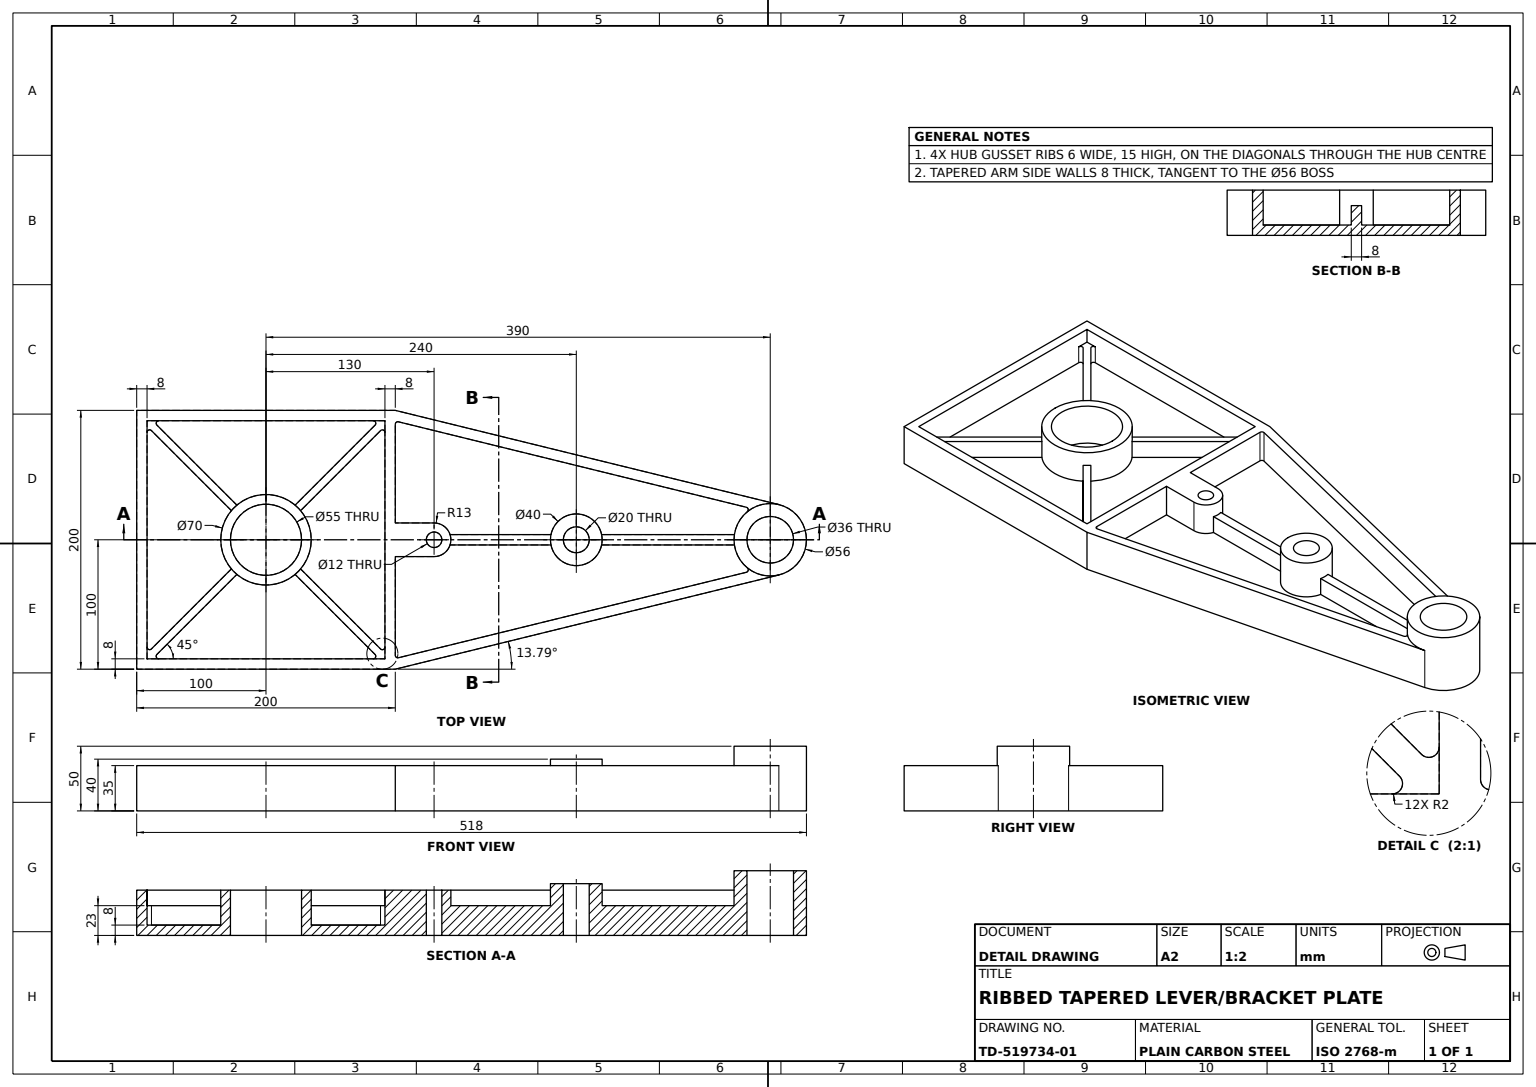
from build123d import *

# Parameters (mm, degrees)
BASE_PLATE_8MM_DEPTH      = 8
PERIMETER_WALL_SKETCH_W   = 200
PERIMETER_WALL_SKETCH_H   = 200
PERIMETER_WALL_SKETCH_W_2 = 184
PERIMETER_WALL_SKETCH_H_2 = 184
PERIMETER_WALL_DEPTH      = 27
CROSS_WALL_DEPTH          = 27
TIP_BOSS_SKETCH_R         = 28
ARM_TIP_BOSS_DEPTH        = 42
ARM_PAD_130X26_DEPTH      = 27
HUB_BOSS_SKETCH_R         = 35
HUB_BOSS_70_DEPTH         = 27
MID_BOSS_SKETCH_R         = 20
MID_ARM_BOSS_40_DEPTH     = 32
HUB_GUSSET_RIBS_4X_DEPTH  = 15
WALL_AND_RIB_FILLETS_R2_R = 2
ARM_RIBS_SKETCH_W         = 8
ARM_RIBS_SKETCH_H         = 265.57093639
ARM_GUSSET_RIBS_DEPTH     = 15
BOSS_BORES_SKETCH_R       = 27.5
BOSS_BORES_SKETCH_R_2     = 6
BOSS_BORES_SKETCH_R_3     = 10
BOSS_BORES_SKETCH_R_4     = 18
BOSS_BORES_DEPTH          = 433.693887177


with BuildPart() as part:
    # Base Plate Sketch → Base Plate 8mm (new body)
    with BuildSketch(Plane(origin=(0, 0, 0), x_dir=(1, 0, 0), z_dir=(0, 1, 0))):
        with BuildLine():
            Line((-100, -100), (100, -100))
            Line((100, -100), (100, 100))
            Line((100, 100), (27.193098987, 396.673482409))
            ThreePointArc((27.193098987, 396.673482409), (0, 418), (-27.193098987, 396.673482409))
            Line((-27.193098987, 396.673482409), (-100, 100))
            Line((-100, 100), (-100, -100))
        make_face()
    extrude(amount=BASE_PLATE_8MM_DEPTH)

    # Perimeter Wall Sketch → Perimeter Wall (add)
    with BuildSketch(Plane(origin=(0, 8, 0), x_dir=(1, 0, 0), z_dir=(0, 1, 0))):
        Rectangle(PERIMETER_WALL_SKETCH_W, PERIMETER_WALL_SKETCH_H)
        Rectangle(PERIMETER_WALL_SKETCH_W_2, PERIMETER_WALL_SKETCH_H_2, mode=Mode.SUBTRACT)
    extrude(amount=PERIMETER_WALL_DEPTH)

    # Cross Wall Sketch → Cross Wall (add)
    with BuildSketch(Plane(origin=(0, 8, 0), x_dir=(1, 0, 0), z_dir=(0, 1, 0))):
        with BuildLine():
            Line((-100, 100), (-27.193098987, 396.673482409))
            ThreePointArc((-27.193098987, 396.673482409), (0, 418), (27.193098987, 396.673482409))
            Line((27.193098987, 396.673482409), (100, 100))
            Line((100, 100), (100, 92))
            Line((100, 92), (-100, 92))
            Line((-100, 92), (-100, 100))
        make_face()
        with BuildLine():
            Line((-89.799328888, 108), (-19.423642134, 394.76677315))
            ThreePointArc((-19.423642134, 394.76677315), (0, 410), (19.423642134, 394.76677315))
            Line((19.423642134, 394.76677315), (89.799328888, 108))
            Line((89.799328888, 108), (91.762615945, 100))
            Line((91.762615945, 100), (-91.762615945, 100))
            Line((-91.762615945, 100), (-89.799328888, 108))
        make_face(mode=Mode.SUBTRACT)
    extrude(amount=CROSS_WALL_DEPTH)

    # Tip Boss Sketch → Arm Tip Boss (add)
    with BuildSketch(Plane(origin=(0, 8, 0), x_dir=(1, 0, 0), z_dir=(0, 1, 0))):
        with Locations(Location((0, 390, 0), (0, 0, 13.788507306))):
            Circle(TIP_BOSS_SKETCH_R)
    extrude(amount=ARM_TIP_BOSS_DEPTH)

    # Arm Pad Sketch → Arm Pad 130x26 (add)
    with BuildSketch(Plane(origin=(0, 8, 0), x_dir=(1, 0, 0), z_dir=(0, 1, 0))):
        with BuildLine():
            Line((-13, 130), (-13, 100))
            Line((-13, 100), (13, 100))
            Line((13, 100), (13, 130))
            ThreePointArc((13, 130), (0, 143), (-13, 130))
        make_face()
    extrude(amount=ARM_PAD_130X26_DEPTH)

    # Hub Boss Sketch → Hub Boss Ø70 (add)
    with BuildSketch(Plane(origin=(0, 8, 0), x_dir=(1, 0, 0), z_dir=(0, 1, 0))):
        with Locations(Location((0, 0, 0), (0, 0, 270))):
            Circle(HUB_BOSS_SKETCH_R)
    extrude(amount=HUB_BOSS_70_DEPTH)

    # Mid Boss Sketch → Mid Arm Boss Ø40 (add)
    with BuildSketch(Plane(origin=(0, 8, 0), x_dir=(1, 0, 0), z_dir=(0, 1, 0))):
        with Locations(Location((0, 240, 0), (0, 0, 270))):
            Circle(MID_BOSS_SKETCH_R)
    extrude(amount=MID_ARM_BOSS_40_DEPTH)

    # Hub Ribs Sketch → Hub Gusset Ribs 4x (add)
    with BuildSketch(Plane(origin=(0, 8, 0), x_dir=(1, 0, 0), z_dir=(0, 1, 0))):
        with BuildLine():
            Line((89.794575879, 94.021945277), (22.544627023, 26.771996421))
            ThreePointArc((22.544627023, 26.771996421), (0.010838319, 34.999998322), (-22.528041932, 26.785953907))
            Line((-22.528041932, 26.785953907), (-89.77930459, 94.037216566))
            Line((-89.77930459, 94.037216566), (-94.021945277, 89.794575879))
            Line((-94.021945277, 89.794575879), (-26.771996421, 22.544627023))
            ThreePointArc((-26.771996421, 22.544627023), (-34.999998322, 0.010838319), (-26.785953907, -22.528041932))
            Line((-26.785953907, -22.528041932), (-94.037216566, -89.77930459))
            Line((-94.037216566, -89.77930459), (-89.794575879, -94.021945277))
            Line((-89.794575879, -94.021945277), (-22.544627023, -26.771996421))
            ThreePointArc((-22.544627023, -26.771996421), (-0.010838319, -34.999998322), (22.528041932, -26.785953907))
            Line((22.528041932, -26.785953907), (89.77930459, -94.037216566))
            Line((89.77930459, -94.037216566), (94.021945277, -89.794575879))
            Line((94.021945277, -89.794575879), (26.771996421, -22.544627023))
            ThreePointArc((26.771996421, -22.544627023), (34.999998322, -0.010838319), (26.785953907, 22.528041932))
            Line((26.785953907, 22.528041932), (94.037216566, 89.77930459))
            Line((94.037216566, 89.77930459), (89.794575879, 94.021945277))
        make_face()
    extrude(amount=HUB_GUSSET_RIBS_4X_DEPTH)

    # Wall and Rib Fillets R2
    wall_and_rib_fillets_r2_edges = [part.edges().sort_by_distance(p)[0] for p in [
        (87.772630602, 15.5, -92),
        (-87.742088024, 15.5, -92),
        (-92, 15.5, -87.772630602),
        (-92, 15.5, 87.742088024),
        (-87.772630602, 15.5, 92),
        (87.742088024, 15.5, 92),
        (92, 15.5, 87.772630602),
        (92, 15.5, -87.742088024),
        (-91.762615945, 21.5, -100),
        (91.762615945, 21.5, -100),
        (24.094106908, 21.5, -375.73556828),
        (-24.094106908, 21.5, -375.73556828),
    ]]
    fillet(wall_and_rib_fillets_r2_edges, radius=WALL_AND_RIB_FILLETS_R2_R)

    # Arm Ribs Sketch → Arm Gusset Ribs (add)
    with BuildSketch(Plane(origin=(0, 8, 0), x_dir=(1, 0, 0), z_dir=(0, 1, 0))):
        with Locations((0, 233.635099789)):
            Rectangle(ARM_RIBS_SKETCH_W, ARM_RIBS_SKETCH_H)
    extrude(amount=ARM_GUSSET_RIBS_DEPTH)

    # Boss Bores Sketch → Boss Bores (cut, through all)
    with BuildSketch(Plane.XZ):
        with Locations(Location((0, 0, 0), (0, 0, 270))):
            Circle(BOSS_BORES_SKETCH_R)
        with Locations(Location((0, -130, 0), (0, 0, 270))):
            Circle(BOSS_BORES_SKETCH_R_2)
        with Locations(Location((0, -240, 0), (0, 0, 270))):
            Circle(BOSS_BORES_SKETCH_R_3)
        with Locations(Location((0, -390, 0), (0, 0, 270))):
            Circle(BOSS_BORES_SKETCH_R_4)
    extrude(amount=-BOSS_BORES_DEPTH, mode=Mode.SUBTRACT)


solid = part.part
